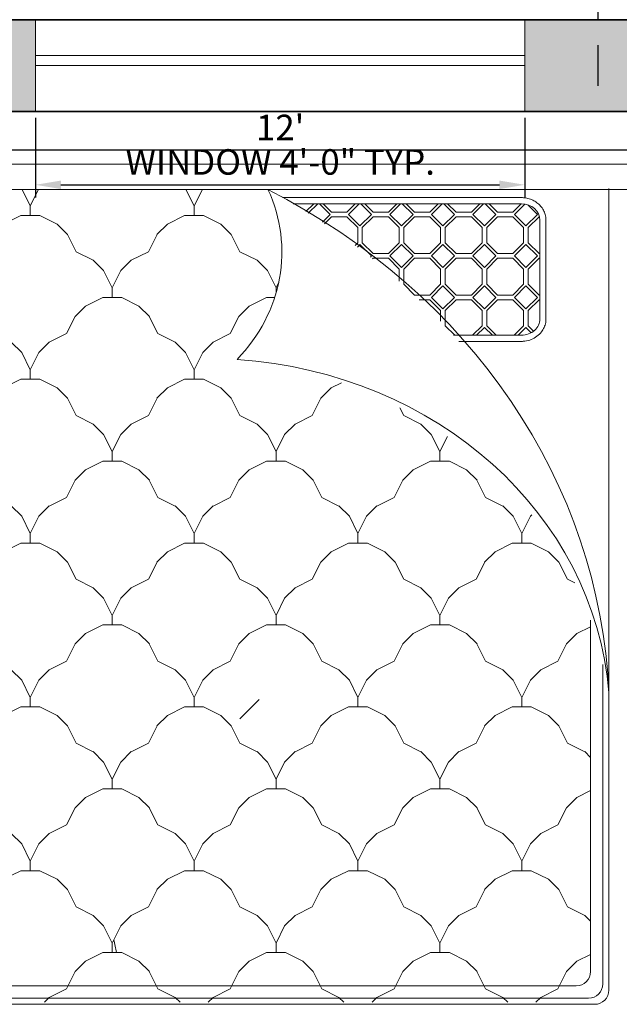
# Model space of a CAD drawing. Units: inches. Extents: x 2901 to 5923, y 918 to 2827.
# Tile 6 of 16: x 4486 to 4544, y 1534 to 1630. Entities that reach past the tile are written whole.
import ezdxf

# ---------------------------------------------------------------- set-up
doc = ezdxf.new("R2010")
doc.units = ezdxf.units.IN
for name, color, linetype, lineweight in [('A-ANNO-DIMS', 2, 'Continuous', 18), ('A-GLAZ', 4, 'Continuous', 18), ('A-WALL-PATT', 7, 'Continuous', 13), ('furniture', 160, 'Continuous', 18), ('walls', 7, 'Continuous', 35)]:
    doc.layers.add(name, color=color, linetype=linetype, lineweight=lineweight)
doc.styles.get("Standard").update_dxf_attribs({"font": 'arial.ttf'})
doc.dimstyles.new('Copy of ISO-25', dxfattribs={"dimtxt": 2.5, "dimasz": 2.5, "dimexe": 1.25, "dimexo": 0.625, "dimtad": 1, "dimdec": 1, "dimlunit": 4, "dimtxsty": 'Standard', "dimcen": 2.5, "dimadec": 0, "dimazin": 0, "dimtfac": 1, "dimtdec": 1, "dimtmove": 0, "dimatfit": 3, "dimfxl": 1, "dimarcsym": 0})

# ---------------------------------------------------------------- blocks, each defined once
blk = doc.blocks.new('A$C029D5C69')
for p, q in [((2.2315, 2.0693), (0.4164, 2.0693)), ((0.4164, 2.0066), (2.2315, 2.0066)), ((0.6869, 1.966), (0.6666, 2.0066)), ((0.7072, 2.0066), (0.6869, 1.966)), ((1.0902, 1.966), (1.0699, 2.0066)), ((1.1106, 2.0066), (1.0902, 1.966)), ((2.1114, 2.0087), (2.1114, 0.0351)), ((0.6869, 1.9425), (0.6869, 1.966)), ((0.6869, 1.9425), (0.6869, 1.966)), ((1.0902, 1.9425), (1.0902, 1.966)), ((1.0902, 1.9425), (1.0902, 1.966)), ((1.8954, 1.9865), (1.3081, 1.9865)), ((1.8954, 1.9713), (1.3339, 1.9713)), ((1.3849, 1.9713), (1.3656, 1.952)), ((1.3945, 1.9713), (1.3714, 1.9483)), ((1.4249, 1.945), (1.3986, 1.9713)), ((1.4288, 1.9507), (1.4081, 1.9713)), ((1.487, 1.9713), (1.4664, 1.9507)), ((1.4966, 1.9713), (1.4703, 1.945)), ((1.527, 1.945), (1.5007, 1.9713)), ((1.5309, 1.9507), (1.5102, 1.9713)), ((1.5891, 1.9713), (1.5685, 1.9507)), ((1.5987, 1.9713), (1.5724, 1.945)), ((1.6291, 1.945), (1.6028, 1.9713)), ((1.633, 1.9507), (1.6123, 1.9713)), ((1.6912, 1.9713), (1.6706, 1.9507)), ((1.7008, 1.9713), (1.6745, 1.945)), ((1.7312, 1.945), (1.7049, 1.9713)), ((1.7351, 1.9507), (1.7144, 1.9713)), ((1.7933, 1.9713), (1.7727, 1.9507)), ((1.8029, 1.9713), (1.7766, 1.945)), ((1.8333, 1.945), (1.807, 1.9713)), ((1.8372, 1.9507), (1.8165, 1.9713)), ((1.8954, 1.9713), (1.8748, 1.9507)), ((1.9043, 1.9707), (1.8787, 1.945)), ((1.9354, 1.945), (1.9114, 1.969)), ((0.6634, 1.9425), (0.621, 1.9213)), ((0.6634, 1.9425), (0.621, 1.9213)), ((0.6869, 1.9425), (0.6634, 1.9425)), ((0.6869, 1.9425), (0.7104, 1.9425)), ((0.7528, 1.9213), (0.7104, 1.9425)), ((0.7528, 1.9213), (0.7104, 1.9425)), ((1.0668, 1.9425), (1.0244, 1.9213)), ((1.0668, 1.9425), (1.0244, 1.9213)), ((1.0902, 1.9425), (1.0668, 1.9425)), ((1.0902, 1.9425), (1.1137, 1.9425)), ((1.1561, 1.9213), (1.1137, 1.9425)), ((1.1561, 1.9213), (1.1137, 1.9425)), ((1.4249, 1.945), (1.4059, 1.926)), ((1.4476, 1.9507), (1.4288, 1.9507)), ((1.4476, 1.9507), (1.4664, 1.9507)), ((1.4986, 1.9167), (1.4703, 1.945)), ((1.527, 1.945), (1.4986, 1.9167)), ((1.5497, 1.9507), (1.5309, 1.9507)), ((1.5497, 1.9507), (1.5685, 1.9507)), ((1.6007, 1.9167), (1.5724, 1.945)), ((1.6291, 1.945), (1.6007, 1.9167)), ((1.6518, 1.9507), (1.633, 1.9507)), ((1.6518, 1.9507), (1.6706, 1.9507)), ((1.7028, 1.9167), (1.6745, 1.945)), ((1.7312, 1.945), (1.7028, 1.9167)), ((1.7539, 1.9507), (1.7351, 1.9507)), ((1.7539, 1.9507), (1.7727, 1.9507)), ((1.8049, 1.9167), (1.7766, 1.945)), ((1.8333, 1.945), (1.8049, 1.9167)), ((1.856, 1.9507), (1.8372, 1.9507)), ((1.856, 1.9507), (1.8748, 1.9507)), ((1.907, 1.9167), (1.8787, 1.945)), ((1.9354, 1.945), (1.907, 1.9167)), ((0.7783, 1.8958), (0.7528, 1.9213)), ((1.0243, 1.9213), (0.9988, 1.8958)), ((1.1816, 1.8958), (1.1561, 1.9213)), ((1.4288, 1.9394), (1.4116, 1.9222)), ((1.4288, 1.9393), (1.4476, 1.9393)), ((1.4664, 1.9393), (1.4476, 1.9393)), ((1.493, 1.9128), (1.4664, 1.9394)), ((1.5309, 1.9394), (1.5043, 1.9128)), ((1.5309, 1.9393), (1.5497, 1.9393)), ((1.5685, 1.9393), (1.5497, 1.9393)), ((1.595, 1.9128), (1.5685, 1.9394)), ((1.633, 1.9394), (1.6064, 1.9128)), ((1.633, 1.9393), (1.6518, 1.9393)), ((1.6706, 1.9393), (1.6518, 1.9393)), ((1.6971, 1.9128), (1.6706, 1.9394)), ((1.7351, 1.9394), (1.7085, 1.9128)), ((1.7351, 1.9393), (1.7539, 1.9393)), ((1.7727, 1.9393), (1.7539, 1.9393)), ((1.7992, 1.9128), (1.7727, 1.9394)), ((1.8372, 1.9394), (1.8106, 1.9128)), ((1.8372, 1.9393), (1.856, 1.9393)), ((1.8748, 1.9393), (1.856, 1.9393)), ((1.9013, 1.9128), (1.8748, 1.9394)), ((1.9393, 1.9394), (1.9127, 1.9128)), ((1.9393, 1.9393), (1.9404, 1.9393)), ((1.9414, 1.688), (1.9414, 1.931)), ((1.9565, 1.688), (1.9565, 1.931)), ((0.7995, 1.8534), (0.7783, 1.8958)), ((0.9989, 1.8958), (0.9777, 1.8534)), ((1.2028, 1.8534), (1.1816, 1.8958)), ((1.493, 1.8752), (1.493, 1.9128)), ((1.5043, 1.8752), (1.5043, 1.9128)), ((1.595, 1.8752), (1.595, 1.9128)), ((1.6064, 1.8752), (1.6064, 1.9128)), ((1.6971, 1.8752), (1.6971, 1.9128)), ((1.7085, 1.8752), (1.7085, 1.9128)), ((1.7992, 1.8752), (1.7992, 1.9128)), ((1.8106, 1.8752), (1.8106, 1.9128)), ((1.9013, 1.8752), (1.9013, 1.9128)), ((1.9127, 1.8752), (1.9127, 1.9128)), ((1.493, 1.8752), (1.4867, 1.869)), ((1.4986, 1.8713), (1.4922, 1.8648)), ((1.527, 1.8429), (1.4986, 1.8713)), ((1.5309, 1.8486), (1.5043, 1.8752)), ((1.595, 1.8752), (1.5685, 1.8486)), ((1.6007, 1.8713), (1.5724, 1.8429)), ((1.6291, 1.8429), (1.6007, 1.8713)), ((1.633, 1.8486), (1.6064, 1.8752)), ((1.6971, 1.8752), (1.6706, 1.8486)), ((1.7028, 1.8713), (1.6745, 1.8429)), ((1.7312, 1.8429), (1.7028, 1.8713)), ((1.7351, 1.8486), (1.7085, 1.8752)), ((1.7992, 1.8752), (1.7727, 1.8486)), ((1.8049, 1.8713), (1.7766, 1.8429)), ((1.8333, 1.8429), (1.8049, 1.8713)), ((1.8372, 1.8486), (1.8106, 1.8752)), ((1.9013, 1.8752), (1.8748, 1.8486)), ((1.907, 1.8713), (1.8787, 1.8429)), ((1.9354, 1.8429), (1.907, 1.8713)), ((1.9393, 1.8486), (1.9127, 1.8752)), ((0.8419, 1.8322), (0.7995, 1.8534)), ((0.8419, 1.8322), (0.7995, 1.8534)), ((0.9777, 1.8534), (0.9353, 1.8322)), ((0.9777, 1.8534), (0.9353, 1.8322)), ((1.2452, 1.8322), (1.2028, 1.8534)), ((1.2452, 1.8322), (1.2028, 1.8534)), ((1.527, 1.8429), (1.5242, 1.8401)), ((1.5497, 1.8486), (1.5309, 1.8486)), ((1.5497, 1.8486), (1.5685, 1.8486)), ((1.6007, 1.8146), (1.5724, 1.8429)), ((1.6291, 1.8429), (1.6007, 1.8146)), ((1.6518, 1.8486), (1.633, 1.8486)), ((1.6518, 1.8486), (1.6706, 1.8486)), ((1.7028, 1.8146), (1.6745, 1.8429)), ((1.7312, 1.8429), (1.7028, 1.8146)), ((1.7539, 1.8486), (1.7351, 1.8486)), ((1.7539, 1.8486), (1.7727, 1.8486)), ((1.8049, 1.8146), (1.7766, 1.8429)), ((1.8333, 1.8429), (1.8049, 1.8146)), ((1.856, 1.8486), (1.8372, 1.8486)), ((1.856, 1.8486), (1.8748, 1.8486)), ((1.907, 1.8146), (1.8787, 1.8429)), ((1.9354, 1.8429), (1.907, 1.8146)), ((1.9414, 1.8486), (1.9393, 1.8486)), ((0.8674, 1.8067), (0.8419, 1.8322)), ((0.9352, 1.8322), (0.9097, 1.8067)), ((1.2707, 1.8067), (1.2452, 1.8322)), ((1.5309, 1.8373), (1.5295, 1.8359)), ((1.5309, 1.8373), (1.5497, 1.8373)), ((1.5685, 1.8373), (1.5497, 1.8373)), ((1.595, 1.8107), (1.5685, 1.8373)), ((1.633, 1.8373), (1.6064, 1.8107)), ((1.633, 1.8373), (1.6518, 1.8373)), ((1.6706, 1.8373), (1.6518, 1.8373)), ((1.6971, 1.8107), (1.6706, 1.8373)), ((1.7351, 1.8373), (1.7085, 1.8107)), ((1.7351, 1.8373), (1.7539, 1.8373)), ((1.7727, 1.8373), (1.7539, 1.8373)), ((1.7992, 1.8107), (1.7727, 1.8373)), ((1.8372, 1.8373), (1.8106, 1.8107)), ((1.8372, 1.8373), (1.856, 1.8373)), ((1.8748, 1.8373), (1.856, 1.8373)), ((1.9013, 1.8107), (1.8748, 1.8373)), ((1.9393, 1.8373), (1.9127, 1.8107)), ((1.9393, 1.8373), (1.9414, 1.8373)), ((0.8886, 1.7643), (0.8674, 1.8067)), ((0.9098, 1.8067), (0.8886, 1.7643)), ((1.2919, 1.7643), (1.2707, 1.8067)), ((1.595, 1.7806), (1.595, 1.8107)), ((1.6064, 1.7731), (1.6064, 1.8107)), ((1.6971, 1.7731), (1.6971, 1.8107)), ((1.7085, 1.7731), (1.7085, 1.8107)), ((1.7992, 1.7731), (1.7992, 1.8107)), ((1.8106, 1.7731), (1.8106, 1.8107)), ((1.9013, 1.7731), (1.9013, 1.8107)), ((1.9127, 1.7731), (1.9127, 1.8107)), ((1.2981, 1.7768), (1.2919, 1.7643)), ((1.633, 1.7465), (1.6064, 1.7731)), ((1.6971, 1.7731), (1.6706, 1.7465)), ((1.7351, 1.7465), (1.7085, 1.7731)), ((1.7992, 1.7731), (1.7727, 1.7465)), ((1.8372, 1.7465), (1.8106, 1.7731)), ((1.9013, 1.7731), (1.8748, 1.7465)), ((1.9393, 1.7465), (1.9127, 1.7731)), ((0.8886, 1.7408), (0.8886, 1.7643)), ((1.2919, 1.7519), (1.2919, 1.7643)), ((1.6518, 1.7465), (1.633, 1.7465)), ((1.6518, 1.7465), (1.6706, 1.7465)), ((1.7028, 1.7692), (1.6745, 1.7408)), ((1.7312, 1.7408), (1.7028, 1.7692)), ((1.7539, 1.7465), (1.7351, 1.7465)), ((1.7539, 1.7465), (1.7727, 1.7465)), ((1.8049, 1.7692), (1.7766, 1.7408)), ((1.8333, 1.7408), (1.8049, 1.7692)), ((1.856, 1.7465), (1.8372, 1.7465)), ((1.856, 1.7465), (1.8748, 1.7465)), ((1.907, 1.7692), (1.8787, 1.7408)), ((1.9354, 1.7408), (1.907, 1.7692)), ((1.9414, 1.7465), (1.9393, 1.7465)), ((0.8651, 1.7408), (0.8227, 1.7196)), ((0.8651, 1.7408), (0.8227, 1.7196)), ((0.912, 1.7408), (0.8651, 1.7408)), ((0.9544, 1.7196), (0.912, 1.7408)), ((0.9544, 1.7196), (0.912, 1.7408)), ((1.2684, 1.7408), (1.226, 1.7196)), ((1.2684, 1.7408), (1.226, 1.7196)), ((1.2885, 1.7408), (1.2684, 1.7408)), ((1.6443, 1.7352), (1.6518, 1.7352)), ((1.6706, 1.7352), (1.6518, 1.7352)), ((1.6971, 1.7086), (1.6706, 1.7352)), ((1.7028, 1.7125), (1.6745, 1.7408)), ((1.7312, 1.7408), (1.7028, 1.7125)), ((1.7351, 1.7352), (1.7085, 1.7086)), ((1.7351, 1.7352), (1.7539, 1.7352)), ((1.7727, 1.7352), (1.7539, 1.7352)), ((1.7992, 1.7086), (1.7727, 1.7352)), ((1.8049, 1.7125), (1.7766, 1.7408)), ((1.8333, 1.7408), (1.8049, 1.7125)), ((1.8372, 1.7352), (1.8106, 1.7086)), ((1.8372, 1.7352), (1.856, 1.7352)), ((1.8748, 1.7352), (1.856, 1.7352)), ((1.9013, 1.7086), (1.8748, 1.7352)), ((1.907, 1.7125), (1.8787, 1.7408)), ((1.9354, 1.7408), (1.907, 1.7125)), ((1.9393, 1.7352), (1.9127, 1.7086)), ((1.9393, 1.7352), (1.9414, 1.7352)), ((0.8227, 1.7196), (0.7972, 1.6941)), ((0.98, 1.6941), (0.9545, 1.7196)), ((1.226, 1.7196), (1.2005, 1.6941)), ((1.6971, 1.682), (1.6971, 1.7086)), ((1.7085, 1.671), (1.7085, 1.7086)), ((1.7992, 1.671), (1.7992, 1.7086)), ((1.8106, 1.671), (1.8106, 1.7086)), ((1.9013, 1.671), (1.9013, 1.7086)), ((1.9127, 1.671), (1.9127, 1.7086)), ((0.7972, 1.6941), (0.776, 1.6517)), ((1.0011, 1.6517), (0.9799, 1.6941)), ((1.2005, 1.6941), (1.1793, 1.6517)), ((0.776, 1.6517), (0.7336, 1.6305)), ((0.776, 1.6517), (0.7336, 1.6305)), ((1.0435, 1.6305), (1.0011, 1.6517)), ((1.0435, 1.6305), (1.0011, 1.6517)), ((1.1793, 1.6517), (1.1369, 1.6305)), ((1.1793, 1.6517), (1.1369, 1.6305)), ((1.7318, 1.6477), (1.7085, 1.671)), ((1.7992, 1.671), (1.7759, 1.6477)), ((1.8049, 1.6671), (1.7855, 1.6477)), ((1.8244, 1.6477), (1.8049, 1.6671)), ((1.8339, 1.6477), (1.8106, 1.671)), ((1.9013, 1.671), (1.878, 1.6477)), ((1.907, 1.6671), (1.8876, 1.6477)), ((1.9202, 1.6539), (1.907, 1.6671)), ((1.926, 1.6577), (1.9127, 1.671)), ((0.6657, 1.605), (0.6402, 1.6305)), ((0.7336, 1.6305), (0.7081, 1.605)), ((1.0691, 1.605), (1.0436, 1.6305)), ((1.1369, 1.6305), (1.1114, 1.605)), ((1.8961, 1.6477), (1.7289, 1.6477)), ((1.8961, 1.6325), (1.7422, 1.6325)), ((0.6869, 1.5626), (0.6657, 1.605)), ((0.7081, 1.605), (0.6869, 1.5626)), ((1.0902, 1.5626), (1.069, 1.605)), ((1.1114, 1.605), (1.0902, 1.5626)), ((0.6869, 1.5392), (0.6869, 1.5626)), ((0.6869, 1.5392), (0.6869, 1.5626)), ((1.0902, 1.5392), (1.0902, 1.5626)), ((1.0902, 1.5392), (1.0902, 1.5626)), ((0.6634, 1.5391), (0.621, 1.5179)), ((0.6634, 1.5391), (0.621, 1.5179)), ((0.6869, 1.5392), (0.6634, 1.5392)), ((0.6869, 1.5392), (0.7104, 1.5392)), ((0.7528, 1.5179), (0.7104, 1.5391)), ((0.7528, 1.5179), (0.7104, 1.5391)), ((1.0668, 1.5391), (1.0244, 1.5179)), ((1.0668, 1.5391), (1.0244, 1.5179)), ((1.0902, 1.5392), (1.0668, 1.5392)), ((1.0902, 1.5392), (1.1137, 1.5392)), ((1.1561, 1.5179), (1.1137, 1.5391)), ((1.1561, 1.5179), (1.1137, 1.5391)), ((1.4534, 1.5308), (1.4277, 1.5179)), ((1.4534, 1.5308), (1.4277, 1.5179)), ((0.7783, 1.4924), (0.7528, 1.5179)), ((1.0243, 1.5179), (0.9988, 1.4924)), ((1.1816, 1.4924), (1.1561, 1.5179)), ((1.4277, 1.5179), (1.4022, 1.4924)), ((0.7995, 1.4501), (0.7783, 1.4925)), ((0.9989, 1.4925), (0.9777, 1.4501)), ((1.2028, 1.4501), (1.1816, 1.4925)), ((1.4022, 1.4925), (1.381, 1.4501)), ((1.6062, 1.4501), (1.5966, 1.4692)), ((0.8419, 1.4288), (0.7995, 1.45)), ((0.8419, 1.4288), (0.7995, 1.45)), ((0.9777, 1.45), (0.9353, 1.4288)), ((0.9777, 1.45), (0.9353, 1.4288)), ((1.2452, 1.4288), (1.2028, 1.45)), ((1.2452, 1.4288), (1.2028, 1.45)), ((1.381, 1.45), (1.3386, 1.4288)), ((1.381, 1.45), (1.3386, 1.4288)), ((1.6486, 1.4288), (1.6062, 1.45)), ((1.6486, 1.4288), (1.6062, 1.45)), ((0.8674, 1.4033), (0.8419, 1.4288)), ((0.9352, 1.4288), (0.9097, 1.4033)), ((1.2707, 1.4033), (1.2452, 1.4288)), ((1.3386, 1.4288), (1.3131, 1.4033)), ((1.6741, 1.4033), (1.6486, 1.4288)), ((0.8886, 1.361), (0.8674, 1.4034)), ((0.9098, 1.4034), (0.8886, 1.361)), ((1.2919, 1.361), (1.2707, 1.4034)), ((1.3131, 1.4034), (1.2919, 1.361)), ((1.6953, 1.361), (1.6741, 1.4034)), ((1.714, 1.3984), (1.6953, 1.361)), ((0.8886, 1.3375), (0.8886, 1.3609)), ((1.2919, 1.3375), (1.2919, 1.3609)), ((1.6953, 1.3375), (1.6953, 1.3609)), ((0.8651, 1.3374), (0.8227, 1.3162)), ((0.8651, 1.3374), (0.8227, 1.3162)), ((0.912, 1.3375), (0.8651, 1.3375)), ((0.9544, 1.3162), (0.912, 1.3374)), ((0.9544, 1.3162), (0.912, 1.3374)), ((1.2684, 1.3374), (1.226, 1.3162)), ((1.2684, 1.3374), (1.226, 1.3162)), ((1.3154, 1.3375), (1.2684, 1.3375)), ((1.3578, 1.3162), (1.3154, 1.3374)), ((1.3578, 1.3162), (1.3154, 1.3374)), ((1.6718, 1.3374), (1.6294, 1.3162)), ((1.6718, 1.3374), (1.6294, 1.3162)), ((1.7187, 1.3375), (1.6718, 1.3375)), ((1.7611, 1.3162), (1.7187, 1.3374)), ((1.7611, 1.3162), (1.7187, 1.3374)), ((0.8227, 1.3163), (0.7972, 1.2908)), ((0.98, 1.2908), (0.9545, 1.3163)), ((1.226, 1.3163), (1.2005, 1.2908)), ((1.3833, 1.2908), (1.3578, 1.3163)), ((1.6294, 1.3163), (1.6039, 1.2908)), ((1.7867, 1.2908), (1.7611, 1.3163)), ((0.7972, 1.2908), (0.776, 1.2484)), ((1.0011, 1.2484), (0.9799, 1.2908)), ((1.2005, 1.2908), (1.1793, 1.2484)), ((1.4045, 1.2484), (1.3833, 1.2908)), ((1.6039, 1.2908), (1.5827, 1.2484)), ((1.8078, 1.2484), (1.7866, 1.2908)), ((0.776, 1.2483), (0.7336, 1.2271)), ((0.776, 1.2483), (0.7336, 1.2271)), ((1.0435, 1.2271), (1.0011, 1.2483)), ((1.0435, 1.2271), (1.0011, 1.2483)), ((1.1793, 1.2483), (1.1369, 1.2271)), ((1.1793, 1.2483), (1.1369, 1.2271)), ((1.4469, 1.2271), (1.4045, 1.2483)), ((1.4469, 1.2271), (1.4045, 1.2483)), ((1.5827, 1.2483), (1.5403, 1.2271)), ((1.5827, 1.2483), (1.5403, 1.2271)), ((1.8502, 1.2271), (1.8078, 1.2483)), ((1.8502, 1.2271), (1.8078, 1.2483)), ((0.6657, 1.2017), (0.6402, 1.2272)), ((0.7336, 1.2272), (0.7081, 1.2017)), ((1.0691, 1.2017), (1.0436, 1.2272)), ((1.1369, 1.2272), (1.1114, 1.2017)), ((1.4724, 1.2017), (1.4469, 1.2272)), ((1.5403, 1.2272), (1.5148, 1.2017)), ((1.8758, 1.2017), (1.8503, 1.2272)), ((0.6869, 1.1593), (0.6657, 1.2017)), ((0.7081, 1.2017), (0.6869, 1.1593)), ((1.0902, 1.1593), (1.069, 1.2017)), ((1.1114, 1.2017), (1.0902, 1.1593)), ((1.4936, 1.1593), (1.4724, 1.2017)), ((1.5148, 1.2017), (1.4936, 1.1593)), ((1.8969, 1.1593), (1.8757, 1.2017)), ((1.9181, 1.2017), (1.8969, 1.1593)), ((1.9215, 1.2051), (1.9181, 1.2017)), ((0.6869, 1.1358), (0.6869, 1.1593)), ((0.6869, 1.1358), (0.6869, 1.1593)), ((1.0902, 1.1358), (1.0902, 1.1593)), ((1.0902, 1.1358), (1.0902, 1.1593)), ((1.4936, 1.1358), (1.4936, 1.1593)), ((1.4936, 1.1358), (1.4936, 1.1593)), ((1.8969, 1.1358), (1.8969, 1.1593)), ((1.8969, 1.1358), (1.8969, 1.1593)), ((0.6634, 1.1358), (0.621, 1.1146)), ((0.6634, 1.1358), (0.621, 1.1146)), ((0.6869, 1.1358), (0.6634, 1.1358)), ((0.6869, 1.1358), (0.7104, 1.1358)), ((0.7528, 1.1146), (0.7104, 1.1358)), ((0.7528, 1.1146), (0.7104, 1.1358)), ((1.0668, 1.1358), (1.0244, 1.1146)), ((1.0668, 1.1358), (1.0244, 1.1146)), ((1.0902, 1.1358), (1.0668, 1.1358)), ((1.0902, 1.1358), (1.1137, 1.1358)), ((1.1561, 1.1146), (1.1137, 1.1358)), ((1.1561, 1.1146), (1.1137, 1.1358)), ((1.4701, 1.1358), (1.4277, 1.1146)), ((1.4701, 1.1358), (1.4277, 1.1146)), ((1.4936, 1.1358), (1.4701, 1.1358)), ((1.4936, 1.1358), (1.5171, 1.1358)), ((1.5595, 1.1146), (1.5171, 1.1358)), ((1.5595, 1.1146), (1.5171, 1.1358)), ((1.8735, 1.1358), (1.8311, 1.1146)), ((1.8735, 1.1358), (1.8311, 1.1146)), ((1.8969, 1.1358), (1.8735, 1.1358)), ((1.8969, 1.1358), (1.9204, 1.1358)), ((1.9628, 1.1146), (1.9204, 1.1358)), ((1.9628, 1.1146), (1.9204, 1.1358)), ((0.7783, 1.0891), (0.7528, 1.1146)), ((1.0243, 1.1146), (0.9988, 1.0891)), ((1.1816, 1.0891), (1.1561, 1.1146)), ((1.4277, 1.1146), (1.4022, 1.0891)), ((1.585, 1.0891), (1.5595, 1.1146)), ((1.831, 1.1146), (1.8055, 1.0891)), ((1.9883, 1.0891), (1.9628, 1.1146)), ((0.7995, 1.0467), (0.7783, 1.0891)), ((0.9989, 1.0891), (0.9777, 1.0467)), ((1.2028, 1.0467), (1.1816, 1.0891)), ((1.4022, 1.0891), (1.381, 1.0467)), ((1.6062, 1.0467), (1.585, 1.0891)), ((1.8056, 1.0891), (1.7844, 1.0467)), ((2.0095, 1.0467), (1.9883, 1.0891)), ((0.8419, 1.0255), (0.7995, 1.0467)), ((0.8419, 1.0255), (0.7995, 1.0467)), ((0.9777, 1.0467), (0.9353, 1.0255)), ((0.9777, 1.0467), (0.9353, 1.0255)), ((1.2452, 1.0255), (1.2028, 1.0467)), ((1.2452, 1.0255), (1.2028, 1.0467)), ((1.381, 1.0467), (1.3386, 1.0255)), ((1.381, 1.0467), (1.3386, 1.0255)), ((1.6486, 1.0255), (1.6062, 1.0467)), ((1.6486, 1.0255), (1.6062, 1.0467)), ((1.7844, 1.0467), (1.742, 1.0255)), ((1.7844, 1.0467), (1.742, 1.0255)), ((2.0276, 1.0376), (2.0095, 1.0467)), ((2.0276, 1.0376), (2.0095, 1.0467)), ((0.8674, 1), (0.8419, 1.0255)), ((0.9352, 1.0255), (0.9097, 1)), ((1.2707, 1), (1.2452, 1.0255)), ((1.3386, 1.0255), (1.3131, 1)), ((1.6741, 1), (1.6486, 1.0255)), ((1.7419, 1.0255), (1.7164, 1)), ((0.8886, 0.9576), (0.8674, 1)), ((0.9098, 1), (0.8886, 0.9576)), ((1.2919, 0.9576), (1.2707, 1)), ((1.3131, 1), (1.2919, 0.9576)), ((1.6953, 0.9576), (1.6741, 1)), ((1.7165, 1), (1.6953, 0.9576)), ((0.8886, 0.9341), (0.8886, 0.9576)), ((1.2919, 0.9341), (1.2919, 0.9576)), ((1.6953, 0.9341), (1.6953, 0.9576)), ((2.066, 0.9457), (2.066, 0.0805)), ((0.8651, 0.9341), (0.8227, 0.9129)), ((0.8651, 0.9341), (0.8227, 0.9129)), ((0.912, 0.9341), (0.8651, 0.9341)), ((0.9544, 0.9129), (0.912, 0.9341)), ((0.9544, 0.9129), (0.912, 0.9341)), ((1.2684, 0.9341), (1.226, 0.9129)), ((1.2684, 0.9341), (1.226, 0.9129)), ((1.3154, 0.9341), (1.2684, 0.9341)), ((1.3578, 0.9129), (1.3154, 0.9341)), ((1.3578, 0.9129), (1.3154, 0.9341)), ((1.6718, 0.9341), (1.6294, 0.9129)), ((1.6718, 0.9341), (1.6294, 0.9129)), ((1.7187, 0.9341), (1.6718, 0.9341)), ((1.7611, 0.9129), (1.7187, 0.9341)), ((1.7611, 0.9129), (1.7187, 0.9341)), ((2.066, 0.9295), (2.0327, 0.9129)), ((2.066, 0.9295), (2.0327, 0.9129)), ((0.8227, 0.9129), (0.7972, 0.8874)), ((0.98, 0.8874), (0.9545, 0.9129)), ((1.226, 0.9129), (1.2005, 0.8874)), ((1.3833, 0.8874), (1.3578, 0.9129)), ((1.6294, 0.9129), (1.6039, 0.8874)), ((1.7867, 0.8874), (1.7611, 0.9129)), ((2.0327, 0.9129), (2.0072, 0.8874)), ((0.7972, 0.8874), (0.776, 0.845)), ((1.0011, 0.845), (0.9799, 0.8874)), ((1.2005, 0.8874), (1.1793, 0.845)), ((1.4045, 0.845), (1.3833, 0.8874)), ((1.6039, 0.8874), (1.5827, 0.845)), ((1.8078, 0.845), (1.7866, 0.8874)), ((2.0072, 0.8874), (1.986, 0.845)), ((0.776, 0.845), (0.7336, 0.8238)), ((0.776, 0.845), (0.7336, 0.8238)), ((1.0435, 0.8238), (1.0011, 0.845)), ((1.0435, 0.8238), (1.0011, 0.845)), ((1.1793, 0.845), (1.1369, 0.8238)), ((1.1793, 0.845), (1.1369, 0.8238)), ((1.4469, 0.8238), (1.4045, 0.845)), ((1.4469, 0.8238), (1.4045, 0.845)), ((1.5827, 0.845), (1.5403, 0.8238)), ((1.5827, 0.845), (1.5403, 0.8238)), ((1.8502, 0.8238), (1.8078, 0.845)), ((1.8502, 0.8238), (1.8078, 0.845)), ((1.986, 0.845), (1.9436, 0.8238)), ((1.986, 0.845), (1.9436, 0.8238)), ((2.0962, 0.8369), (2.0962, 0.0502)), ((0.6657, 0.7983), (0.6402, 0.8238)), ((0.7336, 0.8238), (0.7081, 0.7983)), ((1.0691, 0.7983), (1.0436, 0.8238)), ((1.1369, 0.8238), (1.1114, 0.7983)), ((1.4724, 0.7983), (1.4469, 0.8238)), ((1.5403, 0.8238), (1.5148, 0.7983)), ((1.8758, 0.7983), (1.8503, 0.8238)), ((1.9436, 0.8238), (1.9181, 0.7983)), ((0.6869, 0.7559), (0.6657, 0.7983)), ((0.7081, 0.7983), (0.6869, 0.7559)), ((1.0902, 0.7559), (1.069, 0.7983)), ((1.1114, 0.7983), (1.0902, 0.7559)), ((1.4936, 0.7559), (1.4724, 0.7983)), ((1.5148, 0.7983), (1.4936, 0.7559)), ((1.8969, 0.7559), (1.8757, 0.7983)), ((1.9181, 0.7983), (1.8969, 0.7559)), ((0.6869, 0.7325), (0.6869, 0.7559)), ((0.6869, 0.7325), (0.6869, 0.7559)), ((1.0902, 0.7325), (1.0902, 0.7559)), ((1.0902, 0.7325), (1.0902, 0.7559)), ((1.4936, 0.7325), (1.4936, 0.7559)), ((1.4936, 0.7325), (1.4936, 0.7559)), ((1.8969, 0.7325), (1.8969, 0.7559)), ((1.8969, 0.7325), (1.8969, 0.7559)), ((0.6634, 0.7324), (0.621, 0.7112)), ((0.6634, 0.7324), (0.621, 0.7112)), ((0.6869, 0.7325), (0.6634, 0.7325)), ((0.6869, 0.7325), (0.7104, 0.7325)), ((0.7528, 0.7112), (0.7104, 0.7324)), ((0.7528, 0.7112), (0.7104, 0.7324)), ((1.0668, 0.7324), (1.0244, 0.7112)), ((1.0668, 0.7324), (1.0244, 0.7112)), ((1.0902, 0.7325), (1.0668, 0.7325)), ((1.0902, 0.7325), (1.1137, 0.7325)), ((1.1561, 0.7112), (1.1137, 0.7324)), ((1.1561, 0.7112), (1.1137, 0.7324)), ((1.2024, 0.7028), (1.2503, 0.7507)), ((1.4701, 0.7324), (1.4277, 0.7112)), ((1.4701, 0.7324), (1.4277, 0.7112)), ((1.4936, 0.7325), (1.4701, 0.7325)), ((1.4936, 0.7325), (1.5171, 0.7325)), ((1.5595, 0.7112), (1.5171, 0.7324)), ((1.5595, 0.7112), (1.5171, 0.7324)), ((1.8735, 0.7324), (1.8311, 0.7112)), ((1.8735, 0.7324), (1.8311, 0.7112)), ((1.8969, 0.7325), (1.8735, 0.7325)), ((1.8969, 0.7325), (1.9204, 0.7325)), ((1.9628, 0.7112), (1.9204, 0.7324)), ((1.9628, 0.7112), (1.9204, 0.7324)), ((0.7783, 0.6858), (0.7528, 0.7113)), ((1.0243, 0.7113), (0.9988, 0.6858)), ((1.1816, 0.6858), (1.1561, 0.7113)), ((1.4277, 0.7113), (1.4022, 0.6858)), ((1.585, 0.6858), (1.5595, 0.7113)), ((1.831, 0.7113), (1.8055, 0.6858)), ((1.9883, 0.6858), (1.9628, 0.7113)), ((0.7995, 0.6434), (0.7783, 0.6858)), ((0.9989, 0.6858), (0.9777, 0.6434)), ((1.2028, 0.6434), (1.1816, 0.6858)), ((1.4022, 0.6858), (1.381, 0.6434)), ((1.6062, 0.6434), (1.585, 0.6858)), ((1.8056, 0.6858), (1.7844, 0.6434)), ((2.0095, 0.6434), (1.9883, 0.6858)), ((0.8419, 0.6221), (0.7995, 0.6433)), ((0.8419, 0.6221), (0.7995, 0.6433)), ((0.9777, 0.6433), (0.9353, 0.6221)), ((0.9777, 0.6433), (0.9353, 0.6221)), ((1.2452, 0.6221), (1.2028, 0.6433)), ((1.2452, 0.6221), (1.2028, 0.6433)), ((1.381, 0.6433), (1.3386, 0.6221)), ((1.381, 0.6433), (1.3386, 0.6221)), ((1.6486, 0.6221), (1.6062, 0.6433)), ((1.6486, 0.6221), (1.6062, 0.6433)), ((1.7844, 0.6433), (1.742, 0.6221)), ((1.7844, 0.6433), (1.742, 0.6221)), ((2.0519, 0.6221), (2.0095, 0.6433)), ((2.0519, 0.6221), (2.0095, 0.6433)), ((0.8674, 0.5967), (0.8419, 0.6222)), ((0.9352, 0.6222), (0.9097, 0.5967)), ((1.2707, 0.5967), (1.2452, 0.6222)), ((1.3386, 0.6222), (1.3131, 0.5967)), ((1.6741, 0.5967), (1.6486, 0.6222)), ((1.7419, 0.6222), (1.7164, 0.5967)), ((2.066, 0.6081), (2.0519, 0.6222)), ((0.8886, 0.5543), (0.8674, 0.5967)), ((0.9098, 0.5967), (0.8886, 0.5543)), ((1.2919, 0.5543), (1.2707, 0.5967)), ((1.3131, 0.5967), (1.2919, 0.5543)), ((1.6953, 0.5543), (1.6741, 0.5967)), ((1.7165, 0.5967), (1.6953, 0.5543)), ((0.8886, 0.5308), (0.8886, 0.5543)), ((1.2919, 0.5308), (1.2919, 0.5543)), ((1.6953, 0.5308), (1.6953, 0.5543)), ((0.8227, 0.5096), (0.7972, 0.4841)), ((0.8651, 0.5308), (0.8227, 0.5096)), ((0.8651, 0.5308), (0.8227, 0.5096)), ((0.912, 0.5308), (0.8651, 0.5308)), ((0.9544, 0.5096), (0.912, 0.5308)), ((0.9544, 0.5096), (0.912, 0.5308)), ((0.98, 0.4841), (0.9545, 0.5096)), ((1.226, 0.5096), (1.2005, 0.4841)), ((1.2684, 0.5308), (1.226, 0.5096)), ((1.2684, 0.5308), (1.226, 0.5096)), ((1.3154, 0.5308), (1.2684, 0.5308)), ((1.3578, 0.5096), (1.3154, 0.5308)), ((1.3578, 0.5096), (1.3154, 0.5308)), ((1.3833, 0.4841), (1.3578, 0.5096)), ((1.6294, 0.5096), (1.6039, 0.4841)), ((1.6718, 0.5308), (1.6294, 0.5096)), ((1.6718, 0.5308), (1.6294, 0.5096)), ((1.7187, 0.5308), (1.6718, 0.5308)), ((1.7611, 0.5096), (1.7187, 0.5308)), ((1.7611, 0.5096), (1.7187, 0.5308)), ((1.7867, 0.4841), (1.7611, 0.5096)), ((2.0327, 0.5096), (2.0072, 0.4841)), ((2.066, 0.5262), (2.0327, 0.5096)), ((2.066, 0.5262), (2.0327, 0.5096)), ((0.7972, 0.4841), (0.776, 0.4417)), ((1.0011, 0.4417), (0.9799, 0.4841)), ((1.2005, 0.4841), (1.1793, 0.4417)), ((1.4045, 0.4417), (1.3833, 0.4841)), ((1.6039, 0.4841), (1.5827, 0.4417)), ((1.8078, 0.4417), (1.7866, 0.4841)), ((2.0072, 0.4841), (1.986, 0.4417)), ((0.776, 0.4417), (0.7336, 0.4205)), ((0.776, 0.4417), (0.7336, 0.4205)), ((1.0435, 0.4205), (1.0011, 0.4417)), ((1.0435, 0.4205), (1.0011, 0.4417)), ((1.1793, 0.4417), (1.1369, 0.4205)), ((1.1793, 0.4417), (1.1369, 0.4205)), ((1.4469, 0.4205), (1.4045, 0.4417)), ((1.4469, 0.4205), (1.4045, 0.4417)), ((1.5827, 0.4417), (1.5403, 0.4205)), ((1.5827, 0.4417), (1.5403, 0.4205)), ((1.8502, 0.4205), (1.8078, 0.4417)), ((1.8502, 0.4205), (1.8078, 0.4417)), ((1.986, 0.4417), (1.9436, 0.4205)), ((1.986, 0.4417), (1.9436, 0.4205)), ((0.6657, 0.395), (0.6402, 0.4205)), ((0.7336, 0.4205), (0.7081, 0.395)), ((1.0691, 0.395), (1.0436, 0.4205)), ((1.1369, 0.4205), (1.1114, 0.395)), ((1.4724, 0.395), (1.4469, 0.4205)), ((1.5403, 0.4205), (1.5148, 0.395)), ((1.8758, 0.395), (1.8503, 0.4205)), ((1.9436, 0.4205), (1.9181, 0.395)), ((0.6869, 0.3526), (0.6657, 0.395)), ((0.7081, 0.395), (0.6869, 0.3526)), ((1.0902, 0.3526), (1.069, 0.395)), ((1.1114, 0.395), (1.0902, 0.3526)), ((1.4936, 0.3526), (1.4724, 0.395)), ((1.5148, 0.395), (1.4936, 0.3526)), ((1.8969, 0.3526), (1.8757, 0.395)), ((1.9181, 0.395), (1.8969, 0.3526)), ((0.6869, 0.3291), (0.6869, 0.3526)), ((0.6869, 0.3291), (0.6869, 0.3526)), ((1.0902, 0.3291), (1.0902, 0.3526)), ((1.0902, 0.3291), (1.0902, 0.3526)), ((1.4936, 0.3291), (1.4936, 0.3526)), ((1.4936, 0.3291), (1.4936, 0.3526)), ((1.8969, 0.3291), (1.8969, 0.3526)), ((1.8969, 0.3291), (1.8969, 0.3526)), ((0.6634, 0.3291), (0.621, 0.3079)), ((0.6634, 0.3291), (0.621, 0.3079)), ((0.6869, 0.3291), (0.6634, 0.3291)), ((0.6869, 0.3291), (0.7104, 0.3291)), ((0.7528, 0.3079), (0.7104, 0.3291)), ((0.7528, 0.3079), (0.7104, 0.3291)), ((1.0668, 0.3291), (1.0244, 0.3079)), ((1.0668, 0.3291), (1.0244, 0.3079)), ((1.0902, 0.3291), (1.0668, 0.3291)), ((1.0902, 0.3291), (1.1137, 0.3291)), ((1.1561, 0.3079), (1.1137, 0.3291)), ((1.1561, 0.3079), (1.1137, 0.3291)), ((1.4701, 0.3291), (1.4277, 0.3079)), ((1.4701, 0.3291), (1.4277, 0.3079)), ((1.4936, 0.3291), (1.4701, 0.3291)), ((1.4936, 0.3291), (1.5171, 0.3291)), ((1.5595, 0.3079), (1.5171, 0.3291)), ((1.5595, 0.3079), (1.5171, 0.3291)), ((1.8735, 0.3291), (1.8311, 0.3079)), ((1.8735, 0.3291), (1.8311, 0.3079)), ((1.8969, 0.3291), (1.8735, 0.3291)), ((1.8969, 0.3291), (1.9204, 0.3291)), ((1.9628, 0.3079), (1.9204, 0.3291)), ((1.9628, 0.3079), (1.9204, 0.3291)), ((0.7783, 0.2824), (0.7528, 0.3079)), ((1.0243, 0.3079), (0.9988, 0.2824)), ((1.1816, 0.2824), (1.1561, 0.3079)), ((1.4277, 0.3079), (1.4022, 0.2824)), ((1.585, 0.2824), (1.5595, 0.3079)), ((1.831, 0.3079), (1.8055, 0.2824)), ((1.9883, 0.2824), (1.9628, 0.3079)), ((0.7995, 0.24), (0.7783, 0.2824)), ((0.9989, 0.2824), (0.9777, 0.24)), ((1.2028, 0.24), (1.1816, 0.2824)), ((1.4022, 0.2824), (1.381, 0.24)), ((1.6062, 0.24), (1.585, 0.2824)), ((1.8056, 0.2824), (1.7844, 0.24)), ((2.0095, 0.24), (1.9883, 0.2824)), ((0.8419, 0.2188), (0.7995, 0.24)), ((0.8419, 0.2188), (0.7995, 0.24)), ((0.8674, 0.1933), (0.8419, 0.2188)), ((0.9352, 0.2188), (0.9097, 0.1933)), ((0.9777, 0.24), (0.9353, 0.2188)), ((0.9777, 0.24), (0.9353, 0.2188)), ((1.2452, 0.2188), (1.2028, 0.24)), ((1.2452, 0.2188), (1.2028, 0.24)), ((1.2707, 0.1933), (1.2452, 0.2188)), ((1.3386, 0.2188), (1.3131, 0.1933)), ((1.381, 0.24), (1.3386, 0.2188)), ((1.381, 0.24), (1.3386, 0.2188)), ((1.6486, 0.2188), (1.6062, 0.24)), ((1.6486, 0.2188), (1.6062, 0.24)), ((1.6741, 0.1933), (1.6486, 0.2188)), ((1.7419, 0.2188), (1.7164, 0.1933)), ((1.7844, 0.24), (1.742, 0.2188)), ((1.7844, 0.24), (1.742, 0.2188)), ((2.0519, 0.2188), (2.0095, 0.24)), ((2.0519, 0.2188), (2.0095, 0.24)), ((2.066, 0.2047), (2.0519, 0.2188)), ((0.8886, 0.1509), (0.8674, 0.1933)), ((0.9098, 0.1933), (0.8886, 0.1509)), ((1.2919, 0.1509), (1.2707, 0.1933)), ((1.3131, 0.1933), (1.2919, 0.1509)), ((1.6953, 0.1509), (1.6741, 0.1933)), ((1.7165, 0.1933), (1.6953, 0.1509)), ((0.8886, 0.1275), (0.8886, 0.1509)), ((1.2919, 0.1275), (1.2919, 0.1509)), ((1.6953, 0.1275), (1.6953, 0.1509)), ((0.8651, 0.1274), (0.8227, 0.1062)), ((0.8651, 0.1274), (0.8227, 0.1062)), ((0.912, 0.1275), (0.8651, 0.1275)), ((0.9544, 0.1062), (0.912, 0.1274)), ((0.9544, 0.1062), (0.912, 0.1274)), ((1.2684, 0.1274), (1.226, 0.1062)), ((1.2684, 0.1274), (1.226, 0.1062)), ((1.3154, 0.1275), (1.2684, 0.1275)), ((1.3578, 0.1062), (1.3154, 0.1274)), ((1.3578, 0.1062), (1.3154, 0.1274)), ((1.6718, 0.1274), (1.6294, 0.1062)), ((1.6718, 0.1274), (1.6294, 0.1062)), ((1.7187, 0.1275), (1.6718, 0.1275)), ((1.7611, 0.1062), (1.7187, 0.1274)), ((1.7611, 0.1062), (1.7187, 0.1274)), ((2.066, 0.1228), (2.0327, 0.1062)), ((2.066, 0.1228), (2.0327, 0.1062)), ((0.8227, 0.1062), (0.7972, 0.0807)), ((0.98, 0.0807), (0.9545, 0.1062)), ((1.226, 0.1062), (1.2005, 0.0807)), ((1.3833, 0.0807), (1.3578, 0.1062)), ((1.6294, 0.1062), (1.6039, 0.0807)), ((1.7867, 0.0807), (1.7611, 0.1062)), ((2.0327, 0.1062), (2.0072, 0.0807)), ((0.7972, 0.0808), (0.776, 0.0384)), ((1.0011, 0.0384), (0.9799, 0.0808)), ((1.2005, 0.0808), (1.1793, 0.0384)), ((1.4045, 0.0384), (1.3833, 0.0808)), ((1.6039, 0.0808), (1.5827, 0.0384)), ((1.8078, 0.0384), (1.7866, 0.0808)), ((2.0072, 0.0808), (1.986, 0.0384)), ((2.0309, 0.0454), (0.6056, 0.0454)), ((0.776, 0.0383), (0.7336, 0.0171)), ((0.776, 0.0383), (0.7336, 0.0171)), ((1.0435, 0.0171), (1.0011, 0.0383)), ((1.0435, 0.0171), (1.0011, 0.0383)), ((1.1793, 0.0383), (1.1369, 0.0171)), ((1.1793, 0.0383), (1.1369, 0.0171)), ((1.4469, 0.0171), (1.4045, 0.0383)), ((1.4469, 0.0171), (1.4045, 0.0383)), ((1.5827, 0.0383), (1.5403, 0.0171)), ((1.5827, 0.0383), (1.5403, 0.0171)), ((1.8502, 0.0171), (1.8078, 0.0383)), ((1.8502, 0.0171), (1.8078, 0.0383)), ((1.986, 0.0383), (1.9436, 0.0171)), ((1.986, 0.0383), (1.9436, 0.0171)), ((2.0763, 0), (0.5603, 0)), ((2.0612, 0.0151), (0.5754, 0.0151)), ((0.7336, 0.0171), (0.7215, 0.005)), ((1.0557, 0.005), (1.0436, 0.0171)), ((1.1369, 0.0171), (1.1248, 0.005)), ((1.459, 0.005), (1.4469, 0.0171)), ((1.5403, 0.0171), (1.5282, 0.005)), ((1.8623, 0.005), (1.8503, 0.0171)), ((1.9436, 0.0171), (1.9315, 0.005))]:
    blk.add_line(p, q)
for centre, radius, start, end in [((0.2843, 0.0157), 0.6251, 10.2961, 13.2684), ((2.0309, 0.0805), 0.0351, 270, 0), ((2.0612, 0.0502), 0.0351, 270, 0), ((2.0763, 0.0351), 0.0351, 270, 0)]:
    blk.add_arc(centre, radius, start, end)
for centre, major_axis, ratio, start_param, end_param in [((0.8506, 1.8527), (-0.4556, 0), 0.89, 2.430919, 3.53111), ((0.3667, 0.6698), (1.7398, 0.1668), 0.88072, -0.045073, 0.941433), ((1.8961, 1.931), (-0.0453, 0), 0.89, 3.141593, 4.712389), ((1.8961, 1.688), (-0.0453, 0), 0.89, 1.570796, 3.141593), ((1.0874, 0.6748), (1.021, 0.1213), 0.889348, -0.031673, 1.359628)]:
    blk.add_ellipse(centre, major_axis=major_axis, ratio=ratio, start_param=start_param, end_param=end_param)
for points, knots in [([(1.9565, 1.931), (1.9565, 1.9336), (1.9563, 1.9362), (1.9553, 1.9428), (1.9543, 1.9467), (1.9512, 1.9541), (1.9493, 1.9577), (1.9446, 1.9643), (1.942, 1.9674), (1.936, 1.9729), (1.9327, 1.9753), (1.9257, 1.9795), (1.922, 1.9813), (1.9142, 1.9841), (1.9102, 1.9851), (1.9028, 1.9862), (1.8995, 1.9865), (1.8961, 1.9865)], [3.141593, 3.141593, 3.141593, 3.141593, 3.277614, 3.277614, 3.488082, 3.488082, 3.698551, 3.698551, 3.909019, 3.909019, 4.119488, 4.119488, 4.329956, 4.329956, 4.540424, 4.540424, 4.712389, 4.712389, 4.712389, 4.712389]), ([(1.8961, 1.6325), (1.899, 1.6325), (1.9019, 1.6327), (1.9101, 1.6338), (1.9153, 1.6352), (1.9253, 1.6392), (1.93, 1.6418), (1.9385, 1.6481), (1.9423, 1.6519), (1.9481, 1.6594), (1.9503, 1.663), (1.9537, 1.6707), (1.955, 1.6747), (1.9563, 1.6818), (1.9565, 1.6849), (1.9565, 1.688)], [1.570796, 1.570796, 1.570796, 1.570796, 1.718836, 1.718836, 1.993452, 1.993452, 2.268068, 2.268068, 2.542684, 2.542684, 2.761386, 2.761386, 2.980087, 2.980087, 3.141593, 3.141593, 3.141593, 3.141593])]:
    blk.add_open_spline(points, degree=3, knots=knots)
blk = doc.blocks.new('A$C0D3A6DFA')
blk.add_blockref('A$C029D5C69', (0, 0))
blk = doc.blocks.new('*D36')
at = {"layer": 'A-ANNO-DIMS', "color": 0, "lineweight": -2, "transparency": 16777216}
for p, q in [((4430.068, 1631.022), (4430.068, 1640.2)), ((4892.068, 1631.022), (4892.068, 1640.2)), ((4432.568, 1638.95), (4889.568, 1638.95))]:
    blk.add_line(p, q, dxfattribs=at)
at = {"layer": 'A-ANNO-DIMS', "color": 0, "transparency": 16777216}
for points in [[(4432.568, 1639.367), (4432.568, 1638.533), (4430.068, 1638.95)], [(4889.568, 1639.367), (4889.568, 1638.533), (4892.068, 1638.95)]]:
    blk.add_solid(points, dxfattribs=at)
at = {"layer": 'Defpoints', "color": 0, "transparency": 16777216}
for p in [(4892.068, 1638.95), (4430.068, 1630.397), (4892.068, 1630.397)]:
    blk.add_point(p, dxfattribs=at)
at = {"layer": 'A-ANNO-DIMS', "color": 0, "transparency": 16777216, "insert": (4661.068, 1640.852), "char_height": 2.5, "attachment_point": 5}
blk.add_mtext('38\'-6"', dxfattribs=at)
blk = doc.blocks.new('*D39')
at = {"layer": 'A-ANNO-DIMS', "color": 0, "lineweight": -2, "transparency": 16777216}
for p, q in [((4439.068, 1620.772), (4439.068, 1616.368)), ((4583.068, 1620.772), (4583.068, 1616.368)), ((4441.568, 1617.618), (4580.568, 1617.618))]:
    blk.add_line(p, q, dxfattribs=at)
at = {"layer": 'A-ANNO-DIMS', "color": 0, "transparency": 16777216}
for points in [[(4441.568, 1618.034), (4441.568, 1617.201), (4439.068, 1617.618)], [(4580.568, 1618.034), (4580.568, 1617.201), (4583.068, 1617.618)]]:
    blk.add_solid(points, dxfattribs=at)
at = {"layer": 'Defpoints', "color": 0, "transparency": 16777216}
for p in [(4439.068, 1621.397), (4583.068, 1621.397), (4583.068, 1617.618)]:
    blk.add_point(p, dxfattribs=at)
at = {"layer": 'A-ANNO-DIMS', "color": 0, "transparency": 16777216, "insert": (4511.068, 1619.498), "char_height": 2.5, "attachment_point": 5}
blk.add_mtext("12'", dxfattribs=at)
blk = doc.blocks.new('WIN-48')
for p, q in [((0, 9), (0, 0)), ((48, 0), (48, 9)), ((48, 5.5), (0, 5.5)), ((48, 4.5), (0, 4.5))]:
    blk.add_line(p, q)
blk = doc.blocks.new('*D75')
at = {"layer": 'A-ANNO-DIMS', "color": 0, "lineweight": -2, "transparency": 16777216}
for p, q in [((4487.068, 1620.772), (4487.068, 1612.947)), ((4535.068, 1620.772), (4535.068, 1612.947)), ((4489.568, 1614.197), (4532.568, 1614.197))]:
    blk.add_line(p, q, dxfattribs=at)
at = {"layer": 'A-ANNO-DIMS', "color": 0, "transparency": 16777216}
for points in [[(4489.568, 1614.613), (4489.568, 1613.78), (4487.068, 1614.197)], [(4532.568, 1614.613), (4532.568, 1613.78), (4535.068, 1614.197)]]:
    blk.add_solid(points, dxfattribs=at)
at = {"layer": 'Defpoints', "color": 0, "transparency": 16777216}
for p in [(4487.068, 1621.397), (4535.068, 1621.397), (4535.068, 1614.197)]:
    blk.add_point(p, dxfattribs=at)
at = {"layer": 'A-ANNO-DIMS', "color": 0, "transparency": 16777216, "insert": (4511.068, 1616.115), "char_height": 2.5, "attachment_point": 5}
blk.add_mtext('WINDOW 4\'-0" TYP.', dxfattribs=at)
blk = doc.blocks.new('*D76')
at = {"layer": 'A-ANNO-DIMS', "color": 0, "lineweight": -2, "transparency": 16777216}
for p, q in [((4542.268, 1630.397), (4542.268, 1649.385)), ((4535.693, 1630.397), (4543.518, 1630.397)), ((4542.268, 1623.897), (4542.268, 1627.897)), ((4535.693, 1621.397), (4543.518, 1621.397))]:
    blk.add_line(p, q, dxfattribs=at)
at = {"layer": 'A-ANNO-DIMS', "color": 0, "transparency": 16777216}
for points in [[(4541.852, 1627.897), (4542.685, 1627.897), (4542.268, 1630.397)], [(4541.852, 1623.897), (4542.685, 1623.897), (4542.268, 1621.397)]]:
    blk.add_solid(points, dxfattribs=at)
at = {"layer": 'Defpoints', "color": 0, "transparency": 16777216}
for p in [(4535.068, 1630.397), (4542.268, 1630.397), (4535.068, 1621.397)]:
    blk.add_point(p, dxfattribs=at)
at = {"layer": 'A-ANNO-DIMS', "color": 0, "transparency": 16777216, "insert": (4540.367, 1641.141), "char_height": 2.5, "attachment_point": 5, "rotation": 90}
blk.add_mtext('0\'-9" TYP.', dxfattribs=at)

msp = doc.modelspace()

# ---------------------------------------------------------------- hatches: boundary and pattern name
at = {"layer": 'A-WALL-PATT'}
h = msp.add_hatch(color=256, dxfattribs=at)
h.dxf.hatch_style = 1
h.paths.add_polyline_path([(4439.068, 1447.397), (4583.068, 1447.397), (4583.068, 1340.397), (4589.068, 1340.397), (4589.068, 1453.397), (4589.068, 1455.386), (4583.068, 1455.386), (4583.068, 1453.397), (4439.068, 1453.397), (4439.068, 1501.839), (4430.068, 1501.839), (4430.068, 1399.397), (4439.068, 1399.397)])
h.paths.add_polyline_path([(4439.068, 1621.397), (4487.068, 1621.397), (4487.068, 1630.397), (4430.068, 1630.397), (4430.068, 1561.839), (4439.068, 1561.839)])
h.paths.add_polyline_path([(4630.605, 1630.397), (4535.068, 1630.397), (4535.068, 1621.397), (4583.068, 1621.397), (4583.068, 1495.397), (4589.068, 1495.397), (4637.068, 1495.397), (4637.068, 1501.397), (4589.068, 1501.397), (4589.068, 1621.397), (4630.605, 1621.397)])
h.paths.add_polyline_path([(4892.068, 1630.397), (4690.605, 1630.397), (4690.605, 1621.397), (4733.068, 1621.397), (4733.068, 1564.397), (4739.068, 1564.397), (4739.068, 1621.397), (4883.068, 1621.397), (4883.068, 1528.397), (4739.068, 1528.397), (4733.068, 1528.397), (4733.068, 1501.397), (4685.068, 1501.397), (4685.068, 1495.397), (4739.068, 1495.397), (4739.068, 1519.397), (4787.068, 1519.397), (4787.068, 1423.397), (4739.068, 1423.397), (4739.068, 1456.668), (4733.068, 1456.668), (4733.068, 1340.397), (4739.068, 1340.397), (4739.068, 1417.397), (4787.068, 1417.397), (4793.068, 1417.397), (4793.068, 1423.397), (4793.068, 1519.397), (4883.068, 1519.397), (4883.068, 1482.87), (4892.068, 1482.87)])
h.paths.add_polyline_path([(4892.068, 1458.87), (4883.068, 1458.87), (4883.068, 1423.397), (4823.068, 1423.397), (4823.068, 1417.397), (4883.068, 1417.397), (4883.068, 1363.306), (4892.068, 1363.306)], flags=17)
h.paths.add_polyline_path([(4892.068, 1303.306), (4883.068, 1303.306), (4883.068, 1255.397), (4739.068, 1255.397), (4739.068, 1304.397), (4733.068, 1304.397), (4733.068, 1303.397), (4733.068, 1297.397), (4733.068, 1255.397), (4733.068, 1248.397), (4811.068, 1248.397), (4811.068, 1212.161), (4820.068, 1212.161), (4820.068, 1248.397), (4892.068, 1248.397)])
h.paths.add_polyline_path([(4820.068, 1182.161), (4811.068, 1182.161), (4811.068, 1152.397), (4685.068, 1152.397), (4685.068, 1147.029), (4685.068, 1143.397), (4733.068, 1143.397), (4811.068, 1143.397), (4814.068, 1143.397), (4820.068, 1143.397)])
h.paths.add_polyline_path([(4637.068, 1152.397), (4589.068, 1152.397), (4589.068, 1153.397), (4583.863, 1153.397), (4583.068, 1153.397), (4583.068, 1152.397), (4511.068, 1152.397), (4511.068, 1182.161), (4502.068, 1182.161), (4502.068, 1143.397), (4568.068, 1143.397), (4583.068, 1143.397), (4583.068, 1023.397), (4739.068, 1023.397), (4739.068, 1143.397), (4733.068, 1143.397), (4733.068, 1029.397), (4589.068, 1029.397), (4589.068, 1143.397), (4637.068, 1143.397), (4637.068, 1146.969)])
h.paths.add_polyline_path([(4511.068, 1246.397), (4583.068, 1246.397), (4583.068, 1188.397), (4589.068, 1188.397), (4589.068, 1246.397), (4589.068, 1248.397), (4589.068, 1255.397), (4589.068, 1297.397), (4697.068, 1297.397), (4697.068, 1303.397), (4589.068, 1303.397), (4589.068, 1304.397), (4583.068, 1304.397), (4583.068, 1255.397), (4439.068, 1255.397), (4439.068, 1261.397), (4439.068, 1351.397), (4430.068, 1351.397), (4430.068, 1252.397), (4430.068, 1246.397), (4439.068, 1246.397), (4487.068, 1246.397), (4502.068, 1246.397), (4502.068, 1212.161), (4511.068, 1212.161)])

# ---------------------------------------------------------------- linework, layer by layer
at = {"layer": 'A-GLAZ'}
msp.add_line((4535.068, 1630.397), (4487.068, 1630.397), dxfattribs=at)
at = {"layer": 'walls'}
for p, q in [((4439.068, 1621.397), (4583.068, 1621.397)), ((4583.068, 1621.397), (4535.068, 1621.397))]:
    msp.add_line(p, q, dxfattribs=at)
for points in [[(4892.068, 1630.397), (4430.068, 1630.397), (4430.068, 1252.397)], [(4583.068, 1621.397), (4439.068, 1621.397), (4439.068, 1453.397)]]:
    msp.add_lwpolyline(points, dxfattribs=at)

# ---------------------------------------------------------------- block references
at = {"layer": 'A-GLAZ'}
msp.add_blockref('WIN-48', (4487.068, 1621.397), dxfattribs=at)
at = {"layer": 'furniture', "xscale": 39.84014367312396, "yscale": 39.84014367312396, "zscale": 39.84014367312396}
msp.add_blockref('A$C0D3A6DFA', (4459.192, 1533.796), dxfattribs=at)

# ---------------------------------------------------------------- dimensions: what is measured, and where the dimension line sits
at = {"layer": 'A-ANNO-DIMS'}
dim = msp.add_linear_dim(base=(4542.268, 1630.397), p1=(4535.068, 1621.397), p2=(4535.068, 1630.397), angle=90, text='<> TYP.', dimstyle='Copy of ISO-25', override={"dimdec": 1, "dimlfac": 1, "dimrnd": 0, "dimzin": 1, "dimdsep": 46, "dimlunit": 4, "dimfrac": 2}, dxfattribs=at)
dim.commit()
dim.dimension.update_dxf_attribs({"geometry": '*D76', "text_midpoint": (4540.367, 1641.141)})
for base, p1, p2, picture, middle in [((4892.068, 1638.95), (4430.068, 1630.397), (4892.068, 1630.397), '*D36', (4661.068, 1640.852)), ((4583.068, 1617.618), (4439.068, 1621.397), (4583.068, 1621.397), '*D39', (4511.068, 1619.498))]:
    dim = msp.add_linear_dim(base=base, p1=p1, p2=p2, dimstyle='Copy of ISO-25', override={"dimclrd": 0, "dimclre": 0, "dimclrt": 0}, dxfattribs=at)
    dim.commit()
    dim.dimension.update_dxf_attribs({"geometry": picture, "text_midpoint": middle})
dim = msp.add_linear_dim(base=(4535.068, 1614.197), p1=(4487.068, 1621.397), p2=(4535.068, 1621.397), text='WINDOW <> TYP.', dimstyle='Copy of ISO-25', override={"dimdec": 1, "dimlfac": 1, "dimrnd": 0, "dimzin": 1, "dimdsep": 46, "dimlunit": 4, "dimfrac": 2}, dxfattribs=at)
dim.commit()
dim.dimension.update_dxf_attribs({"geometry": '*D75', "text_midpoint": (4511.068, 1616.115)})

doc.saveas('drawing.dxf')
